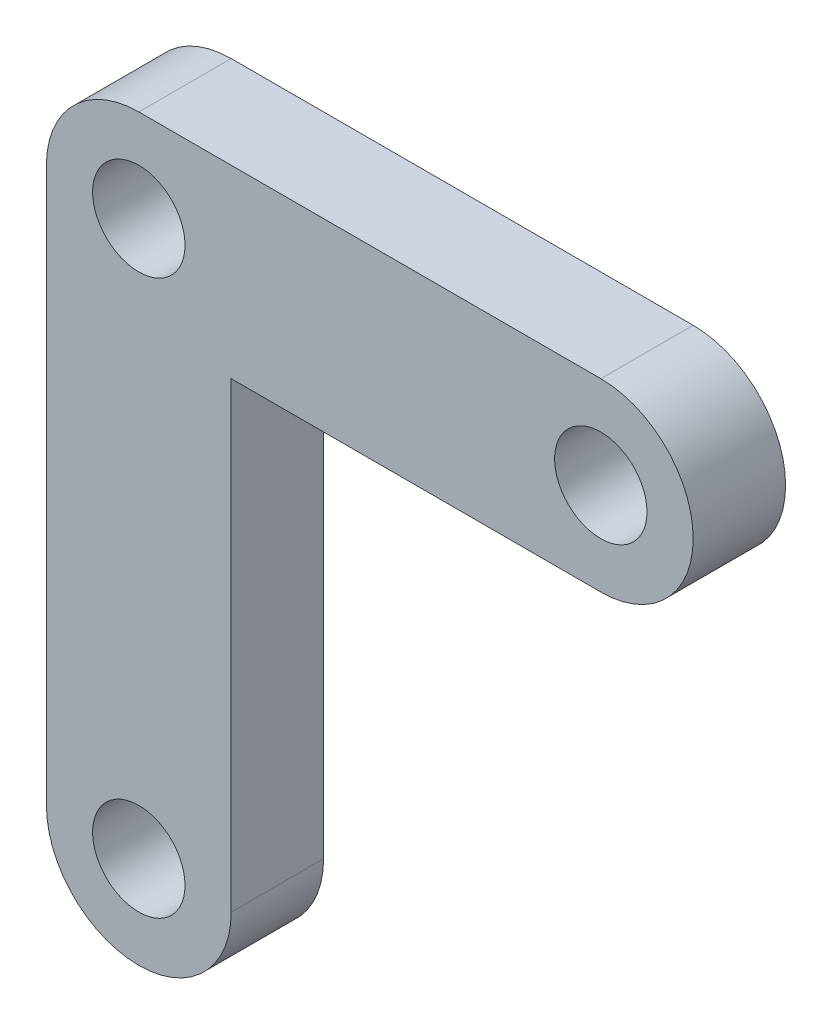
from build123d import *

# Parameters (mm, degrees)
L_LINK_PROFILE_R       = 2.5
L_LINK_PLATE_5MM_DEPTH = 5


with BuildPart() as part:
    # L-Link Profile → L-Link Plate 5mm (new body)
    # profile 1 of 3: a face of its own
    with BuildSketch(Plane.XY):
        with BuildLine():
            Line((25, 5), (0, 5))
            ThreePointArc((0, 5), (3.535533906, 3.535533906), (5, 0))
            Line((5, 0), (5, -5))
            Line((5, -5), (25, -5))
            ThreePointArc((25, -5), (30, 0), (25, 5))
        make_face()
        with Locations((25, 0)):
            Circle(L_LINK_PROFILE_R, mode=Mode.SUBTRACT)
    # profile 2 of 3: a face of its own
    with BuildSketch(Plane.XY):
        with BuildLine():
            Line((-5, 0), (-5, -30))
            ThreePointArc((-5, -30), (0, -35), (5, -30))
            Line((5, -30), (5, -5))
            Line((5, -5), (0, -5))
            ThreePointArc((0, -5), (-3.535533906, -3.535533906), (-5, 0))
        make_face()
        with Locations((0, -30)):
            Circle(L_LINK_PROFILE_R, mode=Mode.SUBTRACT)
    # profile 3 of 3: a face of its own
    with BuildSketch(Plane.XY):
        with BuildLine():
            ThreePointArc((0, 5), (-3.535533906, 3.535533906), (-5, 0))
            ThreePointArc((-5, 0), (-3.535533906, -3.535533906), (0, -5))
            Line((0, -5), (5, -5))
            Line((5, -5), (5, 0))
            ThreePointArc((5, 0), (3.535533906, 3.535533906), (0, 5))
        make_face()
        Circle(L_LINK_PROFILE_R, mode=Mode.SUBTRACT)
    extrude(amount=L_LINK_PLATE_5MM_DEPTH)


solid = part.part
